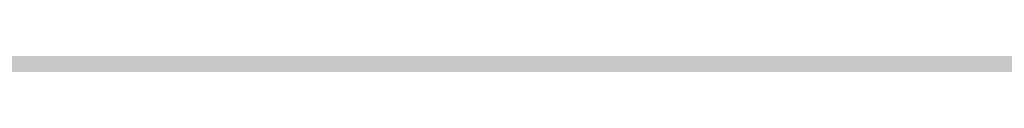
# Model space of a CAD drawing. Units: millimetres. Extents: x 0 to 2267, y 0 to 1823.
# Tile 124 of 256: x 1600.369 to 1605.705, y 1232.256 to 1232.264. Entities that reach past the tile are written whole.
import ezdxf

# ---------------------------------------------------------------- set-up
doc = ezdxf.new("R2010")
doc.units = ezdxf.units.MM
doc.header["$MEASUREMENT"] = 0
doc.layers.add('M-HATC', color=252, linetype='Continuous', lineweight=18)

msp = doc.modelspace()

# ---------------------------------------------------------------- hatches: boundary and pattern name
at = {"layer": 'M-HATC'}
h = msp.add_hatch(color=256, dxfattribs=at)
h.dxf.hatch_style = 1
h.paths.add_polyline_path([(2065.771, 1618.062, 0.236068), (2055.771, 1638.062), (1381.0868, 1638.062, 0.236068), (1371.0868, 1618.062), (1371.0868, 1603.062), (2055.771, 1603.062), (2065.771, 1603.062)])
h.paths.add_polyline_path([(2062.7718, 1550.2964), (2062.7718, 1560.2964), (1374.086, 1560.2964), (1374.086, 1550.2964), (1374.086, 1540.2964), (1384.086, 1540.2964), (1389.086, 1540.2964), (2062.7718, 1540.2964)])
h.paths.add_polyline_path([(1930.9289, 1282.7656), (1505.9289, 1282.7656), (1587.6276, 1235.5968, 0.131652), (1600.1276, 1232.2475), (1836.7302, 1232.2475, 0.131652), (1849.2302, 1235.5968)])
h.paths.add_polyline_path([(1930.9289, 1117.4171), (1905.9289, 1117.4171), (1505.9289, 1117.4171), (1505.9289, 1077.4171), (1930.9289, 1077.4171)])
h = msp.add_hatch(color=256, dxfattribs=at)
h.dxf.hatch_style = 1
h.paths.add_polyline_path([(2055.771, 1603.062), (1381.0868, 1603.062), (1381.0868, 1598.062), (2055.771, 1598.062)])
h.paths.add_polyline_path([(2055.771, 1598.062), (1381.0868, 1598.062), (1381.0868, 1593.062), (2055.771, 1593.062)])
h.paths.add_polyline_path([(2051.3074, 1536.7609), (1385.5504, 1536.7609), (1385.5504, 1526.7609), (1387.5504, 1526.7609), (1388.5366, 1525.0528), (1385.3319, 1521.2335), (1385.3319, 1521.2226), (2050.2542, 1522.7491), (2048.3212, 1525.0528), (2049.3074, 1526.7609), (2051.3074, 1526.7609)])
edge = h.paths.add_edge_path()
edge.add_arc((1847.5345, 1379.1492), 135, 222.603061, 222.890851, ccw=False)
edge.add_line((1748.1663, 1287.7656), (1683.0921, 1287.7656))
edge.add_arc((1583.7239, 1379.1492), 135, 317.109149, 317.396939, ccw=False)
edge.add_arc((1678.9686, 1290.6707), 5, 222.8909, 317.1091, ccw=False)
edge.add_arc((1774.2133, 1379.1492), 135, 222.603061, 222.890851, ccw=False)
edge.add_line((1674.8451, 1287.7656), (1609.7709, 1287.7656))
edge.add_arc((1510.4027, 1379.1492), 135, 317.109149, 317.396939, ccw=False)
edge.add_arc((1605.6474, 1290.6707), 5, 222.8909, 317.1091, ccw=False)
edge.add_arc((1700.8921, 1379.1492), 135, 222.603061, 222.890851, ccw=False)
edge.add_line((1601.5239, 1287.7656), (1536.4497, 1287.7656))
edge.add_arc((1437.0815, 1379.1492), 135, 317.109149, 317.396939, ccw=False)
edge.add_arc((1532.3262, 1290.6707), 5, 222.8909, 317.1091, ccw=False)
edge.add_arc((1627.5709, 1379.1492), 135, 222.603061, 222.890851, ccw=False)
edge.add_line((1528.2027, 1287.7656), (1505.9289, 1287.7656))
edge.add_spline(control_points=[(1505.9289, 1287.7656), (1504.2622, 1287.7656), (1504.2622, 1282.7656), (1505.9289, 1282.7656)], knot_values=[0, 0, 0, 0, 5, 5, 5, 5], degree=3, periodic=0)
edge.add_line((1505.9289, 1282.7656), (1930.9289, 1282.7656))
edge.add_spline(control_points=[(1930.9289, 1282.7656), (1932.5956, 1282.7656), (1932.5956, 1287.7656), (1930.9289, 1287.7656)], knot_values=[0, 0, 0, 0, 5, 5, 5, 5], degree=3, periodic=0)
edge.add_line((1930.9289, 1287.7656), (1903.0557, 1287.7656))
edge.add_arc((1803.6875, 1379.1492), 135, 317.109149, 317.396939, ccw=False)
edge.add_arc((1898.9322, 1290.6707), 5, 222.8909, 317.1091, ccw=False)
edge.add_arc((1994.1769, 1379.1492), 135, 222.603061, 222.890851, ccw=False)
edge.add_line((1894.8087, 1287.7656), (1829.7345, 1287.7656))
edge.add_arc((1730.3663, 1379.1492), 135, 317.109149, 317.396939, ccw=False)
edge.add_arc((1825.611, 1290.6707), 5, 222.8909, 317.1091, ccw=False)
edge.add_arc((1920.8557, 1379.1492), 135, 222.603061, 222.890851, ccw=False)
edge.add_line((1821.4875, 1287.7656), (1756.4133, 1287.7656))
edge.add_arc((1657.0451, 1379.1492), 135, 317.109149, 317.396939, ccw=False)
edge.add_arc((1752.2898, 1290.6707), 5, 222.8909, 317.1091, ccw=False)
edge = h.paths.add_edge_path()
edge.add_spline(control_points=[(1843.4289, 1227.2475), (1845.0956, 1227.2475), (1845.0956, 1232.2475), (1843.4289, 1232.2475)], knot_values=[0, 0, 0, 0, 5, 5, 5, 5], degree=3, periodic=0)
edge.add_line((1843.4289, 1232.2475), (1593.4289, 1232.2475))
edge.add_spline(control_points=[(1593.4289, 1232.2475), (1591.7622, 1232.2475), (1591.7622, 1227.2475), (1593.4289, 1227.2475)], knot_values=[0, 0, 0, 0, 5, 5, 5, 5], degree=3, periodic=0)
edge.add_line((1593.4289, 1227.2475), (1843.4289, 1227.2475))
h.paths.add_polyline_path([(1905.9289, 1127.4171), (1530.9289, 1127.4171, 0.414214), (1520.9289, 1117.4171), (1530.9289, 1117.4171), (1915.9289, 1117.4171, 0.414214)])
edge = h.paths.add_edge_path()
edge.add_arc((1397.0858, 1498.4078), 12.7299, 90.78215, 190.87871, ccw=False)
edge.add_line((1396.912, 1511.1365), (1428.0097, 1511.3488))
edge.add_line((1428.0097, 1511.3488), (1433.0097, 1511.3488))
edge.add_line((1433.0097, 1511.3488), (1434.439, 1511.3488))
edge.add_arc((1419.474, 1498.0804), 20, 41.561, 74.08211)
edge.add_line((1424.9592, 1517.3135), (1399.9351, 1517.2561))
edge.add_spline(control_points=[(1399.9307, 1517.2561), (1399.884, 1517.2131), (1399.8328, 1517.1689), (1399.7774, 1517.1236)], knot_values=[11.567499, 11.567499, 11.567499, 11.567499, 11.814249, 11.814249, 11.814249, 11.814249], degree=3, periodic=0)
edge.add_spline(control_points=[(1399.6328, 1517.0099), (1399.5831, 1516.9721), (1399.5307, 1516.9338), (1399.4759, 1516.8947)], knot_values=[11.167718, 11.167718, 11.167718, 11.167718, 11.365188, 11.365188, 11.365188, 11.365188], degree=3, periodic=0)
edge.add_spline(control_points=[(1399.3398, 1516.8001), (1399.1514, 1516.6719), (1398.9384, 1516.5377), (1398.704, 1516.3994)], knot_values=[10.376405, 10.376405, 10.376405, 10.376405, 11.00994, 11.00994, 11.00994, 11.00994], degree=3, periodic=0)
edge.add_spline(control_points=[(1398.6572, 1516.3719), (1398.5789, 1516.326), (1398.4983, 1516.2797), (1398.4155, 1516.2331)], knot_values=[10.125175, 10.125175, 10.125175, 10.125175, 10.334406, 10.334406, 10.334406, 10.334406], degree=3, periodic=0)
edge.add_spline(control_points=[(1398.2642, 1516.1487), (1398.196, 1516.1111), (1398.1263, 1516.0732), (1398.0555, 1516.0351)], knot_values=[9.832246, 9.832246, 9.832246, 9.832246, 9.999658, 9.999658, 9.999658, 9.999658], degree=3, periodic=0)
edge.add_spline(control_points=[(1397.9987, 1516.0048), (1397.7312, 1515.8621), (1397.446, 1515.7171), (1397.1466, 1515.5714)], knot_values=[9.161808, 9.161808, 9.161808, 9.161808, 9.787769, 9.787769, 9.787769, 9.787769], degree=3, periodic=0)
edge.add_spline(control_points=[(1397.1466, 1515.5714), (1396.8418, 1515.423), (1396.5222, 1515.274), (1396.1914, 1515.1262)], knot_values=[8.524455, 8.524455, 8.524455, 8.524455, 9.161808, 9.161808, 9.161808, 9.161808], degree=3, periodic=0)
edge.add_spline(control_points=[(1396.0777, 1515.0756), (1395.9854, 1515.0348), (1395.8922, 1514.994), (1395.7983, 1514.9534)], knot_values=[8.275193, 8.275193, 8.275193, 8.275193, 8.451726, 8.451726, 8.451726, 8.451726], degree=3, periodic=0)
edge.add_spline(control_points=[(1395.6018, 1514.8691), (1395.4997, 1514.8257), (1395.3968, 1514.7824), (1395.2932, 1514.7394)], knot_values=[7.962917, 7.962917, 7.962917, 7.962917, 8.152764, 8.152764, 8.152764, 8.152764], degree=3, periodic=0)
edge.add_spline(control_points=[(1395.2116, 1514.7057), (1394.8278, 1514.5475), (1394.4345, 1514.3929), (1394.0364, 1514.2442)], knot_values=[7.21254, 7.21254, 7.21254, 7.21254, 7.913148, 7.913148, 7.913148, 7.913148], degree=3, periodic=0)
edge.add_spline(control_points=[(1394.0364, 1514.2442), (1393.7076, 1514.1214), (1393.3754, 1514.0027), (1393.0427, 1513.8895)], knot_values=[6.633733, 6.633733, 6.633733, 6.633733, 7.21254, 7.21254, 7.21254, 7.21254], degree=3, periodic=0)
edge.add_spline(control_points=[(1392.8214, 1513.815), (1392.7198, 1513.7812), (1392.6181, 1513.7479), (1392.5166, 1513.7152)], knot_values=[6.328796, 6.328796, 6.328796, 6.328796, 6.505493, 6.505493, 6.505493, 6.505493], degree=3, periodic=0)
edge.add_spline(control_points=[(1392.5166, 1513.7152), (1392.3187, 1513.6515), (1392.1212, 1513.59), (1391.9244, 1513.531)], knot_values=[5.984605, 5.984605, 5.984605, 5.984605, 6.328796, 6.328796, 6.328796, 6.328796], degree=3, periodic=0)
edge.add_spline(control_points=[(1391.7915, 1513.4915), (1391.3122, 1513.3501), (1390.8384, 1513.2239), (1390.3784, 1513.1171)], knot_values=[5.066697, 5.066697, 5.066697, 5.066697, 5.907055, 5.907055, 5.907055, 5.907055], degree=3, periodic=0)
edge.add_spline(control_points=[(1390.3784, 1513.1171), (1390.1797, 1513.071), (1389.9836, 1513.0284), (1389.7907, 1512.9899)], knot_values=[4.70367, 4.70367, 4.70367, 4.70367, 5.066695, 5.066695, 5.066695, 5.066695], degree=3, periodic=0)
edge.add_spline(control_points=[(1389.422, 1512.9204), (1389.2459, 1512.8892), (1389.0729, 1512.8617), (1388.9036, 1512.8381)], knot_values=[4.130571, 4.130571, 4.130571, 4.130571, 4.469816, 4.469816, 4.469816, 4.469816], degree=3, periodic=0)
edge.add_spline(control_points=[(1388.9036, 1512.8381), (1388.591, 1512.7946), (1388.2911, 1512.7644), (1388.0071, 1512.7494)], knot_values=[3.504031, 3.504031, 3.504031, 3.504031, 4.130571, 4.130571, 4.130571, 4.130571], degree=3, periodic=0)
edge.add_spline(control_points=[(1387.9356, 1512.7459), (1387.8538, 1512.7423), (1387.7733, 1512.74), (1387.6944, 1512.739)], knot_values=[3.268866, 3.268866, 3.268866, 3.268866, 3.451164, 3.451164, 3.451164, 3.451164], degree=3, periodic=0)
edge.add_spline(control_points=[(1387.3351, 1512.7443), (1387.2076, 1512.7499), (1387.0847, 1512.7597), (1386.967, 1512.7739)], knot_values=[2.670686, 2.670686, 2.670686, 2.670686, 2.984, 2.984, 2.984, 2.984], degree=3, periodic=0)
edge.add_spline(control_points=[(1386.8327, 1512.7922), (1386.8209, 1512.7941), (1386.8092, 1512.7959), (1386.7975, 1512.7979)], knot_values=[2.516981, 2.516981, 2.516981, 2.516981, 2.549528, 2.549528, 2.549528, 2.549528], degree=3, periodic=0)
edge.add_spline(control_points=[(1386.4526, 1512.8735), (1386.4257, 1512.881), (1386.3993, 1512.889), (1386.3733, 1512.8972)], knot_values=[2.095869, 2.095869, 2.095869, 2.095869, 2.17941, 2.17941, 2.17941, 2.17941], degree=3, periodic=0)
edge.add_spline(control_points=[(1386.0691, 1513.0189), (1386.0634, 1513.0217), (1386.0577, 1513.0246), (1386.052, 1513.0275)], knot_values=[1.72453, 1.72453, 1.72453, 1.72453, 1.745933, 1.745933, 1.745933, 1.745933], degree=3, periodic=0)
edge.add_arc((1399.474, 1498.0804), 20, 131.82432, 180)
edge.add_arc((1630.3336, 1505.5484), 250.9708, 181.705176, 236.427975)
edge.add_arc((1605.3399, 1483.3044), 218.7822, 238.660829, 243.34961)
edge.add_arc((1647.0911, 1510.3592), 262.8986, 183.129836, 237.853442, ccw=False)
h.paths.add_polyline_path([(1406.5369, 1391.9644, 0.149382), (1491.5506, 1296.4418, -0.129517)], flags=17)
edge = h.paths.add_edge_path()
edge.add_arc((2037.3838, 1498.0804), 20, 0, 48.26587)
edge.add_spline(control_points=[(2050.6973, 1513.0052), (2050.6512, 1512.9847), (2050.6034, 1512.9655), (2050.5539, 1512.9477)], knot_values=[1.835652, 1.835652, 1.835652, 1.835652, 2.000781, 2.000781, 2.000781, 2.000781], degree=3, periodic=0)
edge.add_spline(control_points=[(2050.4616, 1512.9166), (2050.479, 1512.9221), (2050.4963, 1512.9277), (2050.5133, 1512.9335)], knot_values=[2.045477, 2.045477, 2.045477, 2.045477, 2.101389, 2.101389, 2.101389, 2.101389], degree=3, periodic=0)
edge.add_spline(control_points=[(2050.129, 1512.8342), (2050.1984, 1512.8473), (2050.2657, 1512.8623), (2050.3308, 1512.8792)], knot_values=[2.237629, 2.237629, 2.237629, 2.237629, 2.435841, 2.435841, 2.435841, 2.435841], degree=3, periodic=0)
edge.add_spline(control_points=[(2050.0946, 1512.8278), (2050.1061, 1512.8299), (2050.1176, 1512.832), (2050.129, 1512.8342)], knot_values=[2.435841, 2.435841, 2.435841, 2.435841, 2.468321, 2.468321, 2.468321, 2.468321], degree=3, periodic=0)
edge.add_spline(control_points=[(2049.7843, 1512.7851), (2049.8552, 1512.7922), (2049.9243, 1512.8008), (2049.9917, 1512.8109)], knot_values=[2.563852, 2.563852, 2.563852, 2.563852, 2.748541, 2.748541, 2.748541, 2.748541], degree=3, periodic=0)
edge.add_spline(control_points=[(2049.4052, 1512.7617), (2049.5364, 1512.7653), (2049.6629, 1512.773), (2049.7843, 1512.7851)], knot_values=[2.748541, 2.748541, 2.748541, 2.748541, 3.064882, 3.064882, 3.064882, 3.064882], degree=3, periodic=0)
edge.add_spline(control_points=[(2049.1698, 1512.7597), (2049.2336, 1512.7591), (2049.2965, 1512.7594), (2049.3584, 1512.7606)], knot_values=[3.102309, 3.102309, 3.102309, 3.102309, 3.2503, 3.2503, 3.2503, 3.2503], degree=3, periodic=0)
edge.add_spline(control_points=[(2048.8573, 1512.7691), (2048.9638, 1512.7638), (2049.068, 1512.7606), (2049.1698, 1512.7597)], knot_values=[3.2503, 3.2503, 3.2503, 3.2503, 3.486069, 3.486069, 3.486069, 3.486069], degree=3, periodic=0)
edge.add_spline(control_points=[(2048.6924, 1512.7789), (2048.3729, 1512.8009), (2048.0345, 1512.8411), (2047.6817, 1512.897)], knot_values=[3.606429, 3.606429, 3.606429, 3.606429, 4.2989, 4.2989, 4.2989, 4.2989], degree=3, periodic=0)
edge.add_spline(control_points=[(2047.6817, 1512.897), (2047.5458, 1512.9185), (2047.4077, 1512.9424), (2047.2678, 1512.9685)], knot_values=[4.2989, 4.2989, 4.2989, 4.2989, 4.565769, 4.565769, 4.565769, 4.565769], degree=3, periodic=0)
edge.add_spline(control_points=[(2047.2678, 1512.9685), (2047.1449, 1512.9914), (2047.0207, 1513.016), (2046.8951, 1513.0422)], knot_values=[4.565769, 4.565769, 4.565769, 4.565769, 4.799971, 4.799971, 4.799971, 4.799971], degree=3, periodic=0)
edge.add_spline(control_points=[(2046.8951, 1513.0422), (2046.5286, 1513.1188), (2046.1513, 1513.209), (2045.7676, 1513.3107)], knot_values=[4.799971, 4.799971, 4.799971, 4.799971, 5.483718, 5.483718, 5.483718, 5.483718], degree=3, periodic=0)
edge.add_spline(control_points=[(2045.7676, 1513.3107), (2045.3724, 1513.4154), (2044.9704, 1513.5322), (2044.5662, 1513.6588)], knot_values=[5.483718, 5.483718, 5.483718, 5.483718, 6.187866, 6.187866, 6.187866, 6.187866], degree=3, periodic=0)
edge.add_spline(control_points=[(2044.5662, 1513.6588), (2044.4149, 1513.7061), (2044.2633, 1513.7549), (2044.1116, 1513.8048)], knot_values=[6.187866, 6.187866, 6.187866, 6.187866, 6.451551, 6.451551, 6.451551, 6.451551], degree=3, periodic=0)
edge.add_spline(control_points=[(2044.1116, 1513.8048), (2043.9967, 1513.8427), (2043.8817, 1513.8813), (2043.7668, 1513.9205)], knot_values=[6.451551, 6.451551, 6.451551, 6.451551, 6.651434, 6.651434, 6.651434, 6.651434], degree=3, periodic=0)
edge.add_spline(control_points=[(2043.7668, 1513.9205), (2043.3716, 1514.0554), (2042.9774, 1514.1979), (2042.5886, 1514.3458)], knot_values=[6.651434, 6.651434, 6.651434, 6.651434, 7.338879, 7.338879, 7.338879, 7.338879], degree=3, periodic=0)
edge.add_spline(control_points=[(2042.5886, 1514.3458), (2042.1643, 1514.5071), (2041.7465, 1514.6749), (2041.3409, 1514.846)], knot_values=[7.338879, 7.338879, 7.338879, 7.338879, 8.089209, 8.089209, 8.089209, 8.089209], degree=3, periodic=0)
edge.add_spline(control_points=[(2041.3409, 1514.846), (2041.1028, 1514.9465), (2040.869, 1515.0481), (2040.6405, 1515.1502)], knot_values=[8.089209, 8.089209, 8.089209, 8.089209, 8.529587, 8.529587, 8.529587, 8.529587], degree=3, periodic=0)
edge.add_spline(control_points=[(2040.51, 1515.2089), (2040.0824, 1515.4022), (2039.6747, 1515.5971), (2039.295, 1515.7894)], knot_values=[8.613818, 8.613818, 8.613818, 8.613818, 9.44571, 9.44571, 9.44571, 9.44571], degree=3, periodic=0)
edge.add_spline(control_points=[(2039.295, 1515.7894), (2039.0618, 1515.9075), (2038.8391, 1516.0246), (2038.6288, 1516.1398)], knot_values=[9.44571, 9.44571, 9.44571, 9.44571, 9.956404, 9.956404, 9.956404, 9.956404], degree=3, periodic=0)
edge.add_spline(control_points=[(2038.6288, 1516.1398), (2038.5187, 1516.2001), (2038.4121, 1516.2598), (2038.309, 1516.3189)], knot_values=[9.956404, 9.956404, 9.956404, 9.956404, 10.223542, 10.223542, 10.223542, 10.223542], degree=3, periodic=0)
edge.add_spline(control_points=[(2038.309, 1516.3189), (2038.2138, 1516.3735), (2038.1216, 1516.4276), (2038.0328, 1516.481)], knot_values=[10.223542, 10.223542, 10.223542, 10.223542, 10.47051, 10.47051, 10.47051, 10.47051], degree=3, periodic=0)
edge.add_spline(control_points=[(2038.0328, 1516.481), (2037.7855, 1516.6296), (2037.5639, 1516.773), (2037.3722, 1516.909)], knot_values=[10.47051, 10.47051, 10.47051, 10.47051, 11.15767, 11.15767, 11.15767, 11.15767], degree=3, periodic=0)
edge.add_spline(control_points=[(2037.3722, 1516.909), (2037.2789, 1516.9752), (2037.1927, 1517.0396), (2037.1142, 1517.102)], knot_values=[11.15767, 11.15767, 11.15767, 11.15767, 11.49227, 11.49227, 11.49227, 11.49227], degree=3, periodic=0)
edge.add_spline(control_points=[(2036.8564, 1517.3259), (2036.9148, 1517.2692), (2036.9814, 1517.2103), (2037.0557, 1517.1492)], knot_values=[11.577341, 11.577341, 11.577341, 11.577341, 11.91035, 11.91035, 11.91035, 11.91035], degree=3, periodic=0)
edge.add_spline(control_points=[(2036.8074, 1517.3748), (2036.823, 1517.3587), (2036.8393, 1517.3424), (2036.8564, 1517.3259)], knot_values=[11.91035, 11.91035, 11.91035, 11.91035, 12.007402, 12.007402, 12.007402, 12.007402], degree=3, periodic=0)
edge.add_spline(control_points=[(2036.7017, 1517.494), (2036.7104, 1517.483), (2036.7196, 1517.4719), (2036.7291, 1517.4606)], knot_values=[12.184155, 12.184155, 12.184155, 12.184155, 12.255409, 12.255409, 12.255409, 12.255409], degree=3, periodic=0)
edge.add_spline(control_points=[(2036.6159, 1517.6205), (2036.62, 1517.613), (2036.6243, 1517.6055), (2036.6289, 1517.5979)], knot_values=[12.487913, 12.487913, 12.487913, 12.487913, 12.541035, 12.541035, 12.541035, 12.541035], degree=3, periodic=0)
edge.add_spline(control_points=[(2036.5635, 1517.786), (2036.5637, 1517.7794), (2036.5642, 1517.7726), (2036.565, 1517.7658)], knot_values=[12.911761, 12.911761, 12.911761, 12.911761, 12.968286, 12.968286, 12.968286, 12.968286], degree=3, periodic=0)
edge.add_spline(control_points=[(2036.6166, 1517.9304), (2036.6125, 1517.9259), (2036.6086, 1517.9212), (2036.6049, 1517.9165)], knot_values=[13.382527, 13.382527, 13.382527, 13.382527, 13.433791, 13.433791, 13.433791, 13.433791], degree=3, periodic=0)
edge.add_spline(control_points=[(2036.749, 1518.017), (2036.7361, 1518.0116), (2036.7239, 1518.006), (2036.7124, 1518.0002)], knot_values=[13.726299, 13.726299, 13.726299, 13.726299, 13.809928, 13.809928, 13.809928, 13.809928], degree=3, periodic=0)
edge.add_spline(control_points=[(2036.8604, 1518.0528), (2036.8386, 1518.0474), (2036.8181, 1518.0416), (2036.7988, 1518.0353)], knot_values=[13.910887, 13.910887, 13.910887, 13.910887, 14.02153, 14.02153, 14.02153, 14.02153], degree=3, periodic=0)
edge.add_line((2036.9639, 1518.0804), (2032.3838, 1518.0804))
edge.add_line((2032.3838, 1518.0804), (2027.3838, 1518.0804))
edge.add_line((2027.3838, 1518.0804), (2022.3838, 1518.0804))
edge.add_line((2022.3838, 1518.0804), (2017.3838, 1518.0804))
edge.add_arc((2017.3838, 1498.0804), 20, 90, 138.439)
edge.add_line((2002.4188, 1511.3488), (2003.8481, 1511.3488))
edge.add_line((2003.8481, 1511.3488), (2008.8481, 1511.3488))
edge.add_line((2008.8481, 1511.3488), (2039.772, 1511.1377))
edge.add_arc((2039.772, 1498.4078), 12.7299, -10.87871, 90, ccw=False)
edge.add_arc((1789.7668, 1510.3592), 262.8986, 302.146558, 356.870164, ccw=False)
edge.add_arc((1831.5179, 1483.3044), 218.7822, 296.65039, 301.339171)
edge.add_arc((1806.5242, 1505.5484), 250.9708, 303.572025, 358.294824)
h.paths.add_polyline_path([(2030.321, 1391.9644, -0.129517), (1945.3072, 1296.4418, 0.149382)], flags=17)
edge = h.paths.add_edge_path()
edge.add_spline(control_points=[(2037.2464, 1518.0821), (2037.2898, 1518.081), (2037.3355, 1518.0804), (2037.3838, 1518.0804)], knot_values=[0.000012, 0.000012, 0.000012, 0.000012, 0.144754, 0.144754, 0.144754, 0.144754], degree=3, periodic=0)
edge.add_line((2037.3357, 1518.0804), (2037.0096, 1518.0804))
edge.add_spline(control_points=[(2037.0096, 1518.0804), (2036.9822, 1518.0768), (2036.956, 1518.0727), (2036.9312, 1518.0681)], knot_values=[14.13465, 14.13465, 14.13465, 14.13465, 14.247197, 14.247197, 14.247197, 14.247197], degree=3, periodic=0)
edge.add_spline(control_points=[(2036.9312, 1518.0681), (2036.9276, 1518.0674), (2036.9241, 1518.0667), (2036.9205, 1518.0661)], knot_values=[14.118315, 14.118315, 14.118315, 14.118315, 14.13465, 14.13465, 14.13465, 14.13465], degree=3, periodic=0)
edge.add_spline(control_points=[(2036.9205, 1518.0661), (2036.9118, 1518.0644), (2036.9032, 1518.0626), (2036.8948, 1518.0608)], knot_values=[14.078086, 14.078086, 14.078086, 14.078086, 14.118315, 14.118315, 14.118315, 14.118315], degree=3, periodic=0)
edge.add_spline(control_points=[(2036.8948, 1518.0608), (2036.883, 1518.0583), (2036.8716, 1518.0556), (2036.8604, 1518.0528)], knot_values=[14.02153, 14.02153, 14.02153, 14.02153, 14.078086, 14.078086, 14.078086, 14.078086], degree=3, periodic=0)
edge.add_spline(control_points=[(2036.8604, 1518.0528), (2036.8386, 1518.0474), (2036.8181, 1518.0416), (2036.7988, 1518.0353)], knot_values=[13.910887, 13.910887, 13.910887, 13.910887, 14.02153, 14.02153, 14.02153, 14.02153], degree=3, periodic=0)
edge.add_spline(control_points=[(2036.7988, 1518.0353), (2036.7981, 1518.035), (2036.7974, 1518.0348), (2036.7967, 1518.0346)], knot_values=[13.906906, 13.906906, 13.906906, 13.906906, 13.910887, 13.910887, 13.910887, 13.910887], degree=3, periodic=0)
edge.add_spline(control_points=[(2036.7967, 1518.0346), (2036.7882, 1518.0318), (2036.7799, 1518.0289), (2036.7719, 1518.0259)], knot_values=[13.857826, 13.857826, 13.857826, 13.857826, 13.906906, 13.906906, 13.906906, 13.906906], degree=3, periodic=0)
edge.add_spline(control_points=[(2036.7719, 1518.0259), (2036.764, 1518.023), (2036.7564, 1518.02), (2036.749, 1518.017)], knot_values=[13.809928, 13.809928, 13.809928, 13.809928, 13.857826, 13.857826, 13.857826, 13.857826], degree=3, periodic=0)
edge.add_spline(control_points=[(2036.749, 1518.017), (2036.7361, 1518.0116), (2036.7239, 1518.006), (2036.7124, 1518.0002)], knot_values=[13.726299, 13.726299, 13.726299, 13.726299, 13.809928, 13.809928, 13.809928, 13.809928], degree=3, periodic=0)
edge.add_spline(control_points=[(2036.7124, 1518.0002), (2036.7121, 1518), (2036.7118, 1517.9999), (2036.7115, 1517.9997)], knot_values=[13.723993, 13.723993, 13.723993, 13.723993, 13.726299, 13.726299, 13.726299, 13.726299], degree=3, periodic=0)
edge.add_spline(control_points=[(2036.7115, 1517.9997), (2036.7063, 1517.9971), (2036.7013, 1517.9944), (2036.6965, 1517.9917)], knot_values=[13.686536, 13.686536, 13.686536, 13.686536, 13.723993, 13.723993, 13.723993, 13.723993], degree=3, periodic=0)
edge.add_spline(control_points=[(2036.6965, 1517.9917), (2036.6919, 1517.9891), (2036.6874, 1517.9865), (2036.6831, 1517.9839)], knot_values=[13.651251, 13.651251, 13.651251, 13.651251, 13.686536, 13.686536, 13.686536, 13.686536], degree=3, periodic=0)
edge.add_spline(control_points=[(2036.6831, 1517.9839), (2036.6764, 1517.9798), (2036.67, 1517.9757), (2036.6639, 1517.9714)], knot_values=[13.596804, 13.596804, 13.596804, 13.596804, 13.651251, 13.651251, 13.651251, 13.651251], degree=3, periodic=0)
edge.add_spline(control_points=[(2036.6639, 1517.9714), (2036.6636, 1517.9712), (2036.6633, 1517.9709), (2036.6629, 1517.9707)], knot_values=[13.593956, 13.593956, 13.593956, 13.593956, 13.596804, 13.596804, 13.596804, 13.596804], degree=3, periodic=0)
edge.add_spline(control_points=[(2036.6629, 1517.9707), (2036.6603, 1517.9689), (2036.6577, 1517.967), (2036.6552, 1517.9651)], knot_values=[13.570322, 13.570322, 13.570322, 13.570322, 13.593956, 13.593956, 13.593956, 13.593956], degree=3, periodic=0)
edge.add_spline(control_points=[(2036.6552, 1517.9651), (2036.6525, 1517.9631), (2036.6499, 1517.9611), (2036.6474, 1517.9591)], knot_values=[13.545477, 13.545477, 13.545477, 13.545477, 13.570322, 13.570322, 13.570322, 13.570322], degree=3, periodic=0)
edge.add_spline(control_points=[(2036.6474, 1517.9591), (2036.6472, 1517.9589), (2036.6471, 1517.9588), (2036.6469, 1517.9587)], knot_values=[13.543931, 13.543931, 13.543931, 13.543931, 13.545477, 13.545477, 13.545477, 13.545477], degree=3, periodic=0)
edge.add_spline(control_points=[(2036.6469, 1517.9587), (2036.6412, 1517.9541), (2036.6358, 1517.9494), (2036.6307, 1517.9447)], knot_values=[13.488237, 13.488237, 13.488237, 13.488237, 13.543931, 13.543931, 13.543931, 13.543931], degree=3, periodic=0)
edge.add_spline(control_points=[(2036.6307, 1517.9447), (2036.6282, 1517.9423), (2036.6257, 1517.9399), (2036.6233, 1517.9374)], knot_values=[13.460307, 13.460307, 13.460307, 13.460307, 13.488237, 13.488237, 13.488237, 13.488237], degree=3, periodic=0)
edge.add_spline(control_points=[(2036.6233, 1517.9374), (2036.6215, 1517.9356), (2036.6198, 1517.9338), (2036.6181, 1517.932)], knot_values=[13.439712, 13.439712, 13.439712, 13.439712, 13.460307, 13.460307, 13.460307, 13.460307], degree=3, periodic=0)
edge.add_spline(control_points=[(2036.6181, 1517.932), (2036.6176, 1517.9315), (2036.6171, 1517.9309), (2036.6166, 1517.9304)], knot_values=[13.433791, 13.433791, 13.433791, 13.433791, 13.439712, 13.439712, 13.439712, 13.439712], degree=3, periodic=0)
edge.add_spline(control_points=[(2036.6166, 1517.9304), (2036.6125, 1517.9259), (2036.6086, 1517.9212), (2036.6049, 1517.9165)], knot_values=[13.382527, 13.382527, 13.382527, 13.382527, 13.433791, 13.433791, 13.433791, 13.433791], degree=3, periodic=0)
edge.add_spline(control_points=[(2036.6049, 1517.9165), (2036.6026, 1517.9135), (2036.6004, 1517.9104), (2036.5982, 1517.9074)], knot_values=[13.350017, 13.350017, 13.350017, 13.350017, 13.382527, 13.382527, 13.382527, 13.382527], degree=3, periodic=0)
edge.add_spline(control_points=[(2036.5982, 1517.9074), (2036.5972, 1517.9059), (2036.5962, 1517.9043), (2036.5952, 1517.9028)], knot_values=[13.333922, 13.333922, 13.333922, 13.333922, 13.350017, 13.350017, 13.350017, 13.350017], degree=3, periodic=0)
edge.add_spline(control_points=[(2036.5952, 1517.9028), (2036.5945, 1517.9018), (2036.5939, 1517.9009), (2036.5933, 1517.8999)], knot_values=[13.323828, 13.323828, 13.323828, 13.323828, 13.333922, 13.333922, 13.333922, 13.333922], degree=3, periodic=0)
edge.add_spline(control_points=[(2036.5933, 1517.8999), (2036.5905, 1517.8955), (2036.5879, 1517.8909), (2036.5855, 1517.8864)], knot_values=[13.277545, 13.277545, 13.277545, 13.277545, 13.323828, 13.323828, 13.323828, 13.323828], degree=3, periodic=0)
edge.add_spline(control_points=[(2036.5855, 1517.8864), (2036.5836, 1517.8827), (2036.5817, 1517.8789), (2036.5801, 1517.8751)], knot_values=[13.240119, 13.240119, 13.240119, 13.240119, 13.277545, 13.277545, 13.277545, 13.277545], degree=3, periodic=0)
edge.add_spline(control_points=[(2036.5801, 1517.8751), (2036.5795, 1517.8739), (2036.579, 1517.8727), (2036.5785, 1517.8715)], knot_values=[13.228211, 13.228211, 13.228211, 13.228211, 13.240119, 13.240119, 13.240119, 13.240119], degree=3, periodic=0)
edge.add_spline(control_points=[(2036.5785, 1517.8715), (2036.578, 1517.8702), (2036.5774, 1517.869), (2036.5769, 1517.8677)], knot_values=[13.215717, 13.215717, 13.215717, 13.215717, 13.228211, 13.228211, 13.228211, 13.228211], degree=3, periodic=0)
edge.add_spline(control_points=[(2036.5769, 1517.8677), (2036.5755, 1517.864), (2036.5741, 1517.8603), (2036.5729, 1517.8565)], knot_values=[13.179847, 13.179847, 13.179847, 13.179847, 13.215717, 13.215717, 13.215717, 13.215717], degree=3, periodic=0)
edge.add_spline(control_points=[(2036.5729, 1517.8565), (2036.5713, 1517.8515), (2036.5699, 1517.8464), (2036.5687, 1517.8413)], knot_values=[13.132017, 13.132017, 13.132017, 13.132017, 13.179847, 13.179847, 13.179847, 13.179847], degree=3, periodic=0)
edge.add_spline(control_points=[(2036.5687, 1517.8413), (2036.5684, 1517.8402), (2036.5682, 1517.8392), (2036.568, 1517.8382)], knot_values=[13.122482, 13.122482, 13.122482, 13.122482, 13.132017, 13.132017, 13.132017, 13.132017], degree=3, periodic=0)
edge.add_spline(control_points=[(2036.568, 1517.8382), (2036.5676, 1517.8363), (2036.5672, 1517.8345), (2036.5669, 1517.8327)], knot_values=[13.105592, 13.105592, 13.105592, 13.105592, 13.122482, 13.122482, 13.122482, 13.122482], degree=3, periodic=0)
edge.add_spline(control_points=[(2036.5669, 1517.8327), (2036.5662, 1517.8292), (2036.5657, 1517.8257), (2036.5652, 1517.8222)], knot_values=[13.074063, 13.074063, 13.074063, 13.074063, 13.105592, 13.105592, 13.105592, 13.105592], degree=3, periodic=0)
edge.add_spline(control_points=[(2036.5652, 1517.8222), (2036.5652, 1517.8222), (2036.5652, 1517.8222), (2036.5652, 1517.8222)], knot_values=[13.074043, 13.074043, 13.074043, 13.074043, 13.074063, 13.074063, 13.074063, 13.074063], degree=3, periodic=0)
edge.add_spline(control_points=[(2036.5652, 1517.8222), (2036.5644, 1517.8164), (2036.5639, 1517.8106), (2036.5636, 1517.8046)], knot_values=[13.021884, 13.021884, 13.021884, 13.021884, 13.074043, 13.074043, 13.074043, 13.074043], degree=3, periodic=0)
edge.add_spline(control_points=[(2036.5636, 1517.8046), (2036.5636, 1517.804), (2036.5636, 1517.8034), (2036.5635, 1517.8028)], knot_values=[13.01674, 13.01674, 13.01674, 13.01674, 13.021884, 13.021884, 13.021884, 13.021884], degree=3, periodic=0)
edge.add_spline(control_points=[(2036.5635, 1517.8028), (2036.5634, 1517.8005), (2036.5634, 1517.7982), (2036.5634, 1517.7958)], knot_values=[12.996438, 12.996438, 12.996438, 12.996438, 13.01674, 13.01674, 13.01674, 13.01674], degree=3, periodic=0)
edge.add_spline(control_points=[(2036.5634, 1517.7958), (2036.5633, 1517.7926), (2036.5634, 1517.7893), (2036.5635, 1517.786)], knot_values=[12.968286, 12.968286, 12.968286, 12.968286, 12.996438, 12.996438, 12.996438, 12.996438], degree=3, periodic=0)
edge.add_spline(control_points=[(2036.5635, 1517.786), (2036.5637, 1517.7794), (2036.5642, 1517.7726), (2036.565, 1517.7658)], knot_values=[12.911761, 12.911761, 12.911761, 12.911761, 12.968286, 12.968286, 12.968286, 12.968286], degree=3, periodic=0)
edge.add_spline(control_points=[(2036.565, 1517.7658), (2036.565, 1517.7657), (2036.565, 1517.7656), (2036.565, 1517.7656)], knot_values=[12.911017, 12.911017, 12.911017, 12.911017, 12.911761, 12.911761, 12.911761, 12.911761], degree=3, periodic=0)
edge.add_spline(control_points=[(2036.565, 1517.7656), (2036.5654, 1517.7625), (2036.5658, 1517.7593), (2036.5663, 1517.7562)], knot_values=[12.88528, 12.88528, 12.88528, 12.88528, 12.911017, 12.911017, 12.911017, 12.911017], degree=3, periodic=0)
edge.add_spline(control_points=[(2036.5663, 1517.7562), (2036.5667, 1517.7534), (2036.5672, 1517.7506), (2036.5677, 1517.7478)], knot_values=[12.862519, 12.862519, 12.862519, 12.862519, 12.88528, 12.88528, 12.88528, 12.88528], degree=3, periodic=0)
edge.add_spline(control_points=[(2036.5677, 1517.7478), (2036.5678, 1517.7474), (2036.5679, 1517.7469), (2036.568, 1517.7465)], knot_values=[12.858885, 12.858885, 12.858885, 12.858885, 12.862519, 12.862519, 12.862519, 12.862519], degree=3, periodic=0)
edge.add_spline(control_points=[(2036.568, 1517.7465), (2036.5692, 1517.7399), (2036.5707, 1517.7332), (2036.5724, 1517.7264)], knot_values=[12.8053, 12.8053, 12.8053, 12.8053, 12.858885, 12.858885, 12.858885, 12.858885], degree=3, periodic=0)
edge.add_spline(control_points=[(2036.5724, 1517.7264), (2036.5734, 1517.7226), (2036.5745, 1517.7187), (2036.5756, 1517.7149)], knot_values=[12.775176, 12.775176, 12.775176, 12.775176, 12.8053, 12.8053, 12.8053, 12.8053], degree=3, periodic=0)
edge.add_spline(control_points=[(2036.5756, 1517.7149), (2036.5763, 1517.7125), (2036.577, 1517.7102), (2036.5778, 1517.7078)], knot_values=[12.756759, 12.756759, 12.756759, 12.756759, 12.775176, 12.775176, 12.775176, 12.775176], degree=3, periodic=0)
edge.add_spline(control_points=[(2036.5778, 1517.7078), (2036.5781, 1517.7067), (2036.5784, 1517.7057), (2036.5787, 1517.7047)], knot_values=[12.748742, 12.748742, 12.748742, 12.748742, 12.756759, 12.756759, 12.756759, 12.756759], degree=3, periodic=0)
edge.add_spline(control_points=[(2036.5787, 1517.7047), (2036.5808, 1517.6983), (2036.5831, 1517.6919), (2036.5856, 1517.6854)], knot_values=[12.69959, 12.69959, 12.69959, 12.69959, 12.748742, 12.748742, 12.748742, 12.748742], degree=3, periodic=0)
edge.add_spline(control_points=[(2036.5856, 1517.6854), (2036.5876, 1517.68), (2036.5898, 1517.6746), (2036.5921, 1517.6692)], knot_values=[12.659038, 12.659038, 12.659038, 12.659038, 12.69959, 12.69959, 12.69959, 12.69959], degree=3, periodic=0)
edge.add_spline(control_points=[(2036.5921, 1517.6692), (2036.594, 1517.6648), (2036.5959, 1517.6605), (2036.5979, 1517.6561)], knot_values=[12.626806, 12.626806, 12.626806, 12.626806, 12.659038, 12.659038, 12.659038, 12.659038], degree=3, periodic=0)
edge.add_spline(control_points=[(2036.5979, 1517.6561), (2036.5984, 1517.6551), (2036.5989, 1517.6541), (2036.5993, 1517.6531)], knot_values=[12.619394, 12.619394, 12.619394, 12.619394, 12.626806, 12.626806, 12.626806, 12.626806], degree=3, periodic=0)
edge.add_spline(control_points=[(2036.5993, 1517.6531), (2036.6043, 1517.6424), (2036.6099, 1517.6315), (2036.6159, 1517.6205)], knot_values=[12.541039, 12.541039, 12.541039, 12.541039, 12.619394, 12.619394, 12.619394, 12.619394], degree=3, periodic=0)
edge.add_spline(control_points=[(2036.6159, 1517.6205), (2036.6159, 1517.6205), (2036.6159, 1517.6205), (2036.6159, 1517.6205)], knot_values=[12.541035, 12.541035, 12.541035, 12.541035, 12.541039, 12.541039, 12.541039, 12.541039], degree=3, periodic=0)
edge.add_spline(control_points=[(2036.6159, 1517.6205), (2036.62, 1517.613), (2036.6243, 1517.6055), (2036.6289, 1517.5979)], knot_values=[12.487913, 12.487913, 12.487913, 12.487913, 12.541035, 12.541035, 12.541035, 12.541035], degree=3, periodic=0)
edge.add_spline(control_points=[(2036.6289, 1517.5979), (2036.6326, 1517.5916), (2036.6365, 1517.5853), (2036.6406, 1517.5789)], knot_values=[12.443982, 12.443982, 12.443982, 12.443982, 12.487913, 12.487913, 12.487913, 12.487913], degree=3, periodic=0)
edge.add_spline(control_points=[(2036.6406, 1517.5789), (2036.6414, 1517.5776), (2036.6423, 1517.5763), (2036.6431, 1517.5749)], knot_values=[12.434996, 12.434996, 12.434996, 12.434996, 12.443982, 12.443982, 12.443982, 12.443982], degree=3, periodic=0)
edge.add_spline(control_points=[(2036.6431, 1517.5749), (2036.6531, 1517.5596), (2036.6639, 1517.5439), (2036.6756, 1517.528)], knot_values=[12.329647, 12.329647, 12.329647, 12.329647, 12.434996, 12.434996, 12.434996, 12.434996], degree=3, periodic=0)
edge.add_spline(control_points=[(2036.6756, 1517.528), (2036.6839, 1517.5168), (2036.6925, 1517.5055), (2036.7017, 1517.494)], knot_values=[12.255409, 12.255409, 12.255409, 12.255409, 12.329647, 12.329647, 12.329647, 12.329647], degree=3, periodic=0)
edge.add_spline(control_points=[(2036.7017, 1517.494), (2036.7104, 1517.483), (2036.7196, 1517.4719), (2036.7291, 1517.4606)], knot_values=[12.184155, 12.184155, 12.184155, 12.184155, 12.255409, 12.255409, 12.255409, 12.255409], degree=3, periodic=0)
edge.add_spline(control_points=[(2036.7291, 1517.4606), (2036.7436, 1517.4435), (2036.759, 1517.4262), (2036.7753, 1517.4085)], knot_values=[12.075961, 12.075961, 12.075961, 12.075961, 12.184155, 12.184155, 12.184155, 12.184155], degree=3, periodic=0)
edge.add_spline(control_points=[(2036.7753, 1517.4085), (2036.7763, 1517.4075), (2036.7773, 1517.4064), (2036.7783, 1517.4054)], knot_values=[12.069502, 12.069502, 12.069502, 12.069502, 12.075961, 12.075961, 12.075961, 12.075961], degree=3, periodic=0)
edge.add_spline(control_points=[(2036.7783, 1517.4054), (2036.7877, 1517.3953), (2036.7974, 1517.385), (2036.8074, 1517.3748)], knot_values=[12.007402, 12.007402, 12.007402, 12.007402, 12.069502, 12.069502, 12.069502, 12.069502], degree=3, periodic=0)
edge.add_spline(control_points=[(2036.8074, 1517.3748), (2036.823, 1517.3587), (2036.8393, 1517.3424), (2036.8564, 1517.3259)], knot_values=[11.91035, 11.91035, 11.91035, 11.91035, 12.007402, 12.007402, 12.007402, 12.007402], degree=3, periodic=0)
edge.add_spline(control_points=[(2036.8564, 1517.3259), (2036.9148, 1517.2692), (2036.9814, 1517.2103), (2037.0557, 1517.1492)], knot_values=[11.577341, 11.577341, 11.577341, 11.577341, 11.91035, 11.91035, 11.91035, 11.91035], degree=3, periodic=0)
edge.add_spline(control_points=[(2037.0557, 1517.1492), (2037.0747, 1517.1336), (2037.0942, 1517.1179), (2037.1142, 1517.102)], knot_values=[11.49227, 11.49227, 11.49227, 11.49227, 11.577341, 11.577341, 11.577341, 11.577341], degree=3, periodic=0)
edge.add_spline(control_points=[(2037.1142, 1517.102), (2037.1927, 1517.0396), (2037.2789, 1516.9752), (2037.3722, 1516.909)], knot_values=[11.15767, 11.15767, 11.15767, 11.15767, 11.49227, 11.49227, 11.49227, 11.49227], degree=3, periodic=0)
edge.add_spline(control_points=[(2037.3722, 1516.909), (2037.5639, 1516.773), (2037.7855, 1516.6296), (2038.0328, 1516.481)], knot_values=[10.47051, 10.47051, 10.47051, 10.47051, 11.15767, 11.15767, 11.15767, 11.15767], degree=3, periodic=0)
edge.add_spline(control_points=[(2038.0328, 1516.481), (2038.1216, 1516.4276), (2038.2138, 1516.3735), (2038.309, 1516.3189)], knot_values=[10.223542, 10.223542, 10.223542, 10.223542, 10.47051, 10.47051, 10.47051, 10.47051], degree=3, periodic=0)
edge.add_spline(control_points=[(2038.309, 1516.3189), (2038.4121, 1516.2598), (2038.5187, 1516.2001), (2038.6288, 1516.1398)], knot_values=[9.956404, 9.956404, 9.956404, 9.956404, 10.223542, 10.223542, 10.223542, 10.223542], degree=3, periodic=0)
edge.add_spline(control_points=[(2038.6288, 1516.1398), (2038.8391, 1516.0246), (2039.0618, 1515.9075), (2039.295, 1515.7894)], knot_values=[9.44571, 9.44571, 9.44571, 9.44571, 9.956404, 9.956404, 9.956404, 9.956404], degree=3, periodic=0)
edge.add_spline(control_points=[(2039.295, 1515.7894), (2039.6747, 1515.5971), (2040.0824, 1515.4022), (2040.51, 1515.2089)], knot_values=[8.613818, 8.613818, 8.613818, 8.613818, 9.44571, 9.44571, 9.44571, 9.44571], degree=3, periodic=0)
edge.add_spline(control_points=[(2040.51, 1515.2089), (2040.5533, 1515.1893), (2040.5968, 1515.1697), (2040.6405, 1515.1502)], knot_values=[8.529587, 8.529587, 8.529587, 8.529587, 8.613818, 8.613818, 8.613818, 8.613818], degree=3, periodic=0)
edge.add_spline(control_points=[(2040.6405, 1515.1502), (2040.869, 1515.0481), (2041.1028, 1514.9465), (2041.3409, 1514.846)], knot_values=[8.089209, 8.089209, 8.089209, 8.089209, 8.529587, 8.529587, 8.529587, 8.529587], degree=3, periodic=0)
edge.add_spline(control_points=[(2041.3409, 1514.846), (2041.7465, 1514.6749), (2042.1643, 1514.5071), (2042.5886, 1514.3458)], knot_values=[7.338879, 7.338879, 7.338879, 7.338879, 8.089209, 8.089209, 8.089209, 8.089209], degree=3, periodic=0)
edge.add_spline(control_points=[(2042.5886, 1514.3458), (2042.9774, 1514.1979), (2043.3716, 1514.0554), (2043.7668, 1513.9205)], knot_values=[6.651434, 6.651434, 6.651434, 6.651434, 7.338879, 7.338879, 7.338879, 7.338879], degree=3, periodic=0)
edge.add_spline(control_points=[(2043.7668, 1513.9205), (2043.8817, 1513.8813), (2043.9967, 1513.8427), (2044.1116, 1513.8048)], knot_values=[6.451551, 6.451551, 6.451551, 6.451551, 6.651434, 6.651434, 6.651434, 6.651434], degree=3, periodic=0)
edge.add_spline(control_points=[(2044.1116, 1513.8048), (2044.2633, 1513.7549), (2044.4149, 1513.7061), (2044.5662, 1513.6588)], knot_values=[6.187866, 6.187866, 6.187866, 6.187866, 6.451551, 6.451551, 6.451551, 6.451551], degree=3, periodic=0)
edge.add_spline(control_points=[(2044.5662, 1513.6588), (2044.9704, 1513.5322), (2045.3724, 1513.4154), (2045.7676, 1513.3107)], knot_values=[5.483718, 5.483718, 5.483718, 5.483718, 6.187866, 6.187866, 6.187866, 6.187866], degree=3, periodic=0)
edge.add_spline(control_points=[(2045.7676, 1513.3107), (2046.1513, 1513.209), (2046.5286, 1513.1188), (2046.8951, 1513.0422)], knot_values=[4.799971, 4.799971, 4.799971, 4.799971, 5.483718, 5.483718, 5.483718, 5.483718], degree=3, periodic=0)
edge.add_spline(control_points=[(2046.8951, 1513.0422), (2047.0207, 1513.016), (2047.1449, 1512.9914), (2047.2678, 1512.9685)], knot_values=[4.565769, 4.565769, 4.565769, 4.565769, 4.799971, 4.799971, 4.799971, 4.799971], degree=3, periodic=0)
edge.add_spline(control_points=[(2047.2678, 1512.9685), (2047.4077, 1512.9424), (2047.5458, 1512.9185), (2047.6817, 1512.897)], knot_values=[4.2989, 4.2989, 4.2989, 4.2989, 4.565769, 4.565769, 4.565769, 4.565769], degree=3, periodic=0)
edge.add_spline(control_points=[(2047.6817, 1512.897), (2048.0345, 1512.8411), (2048.3729, 1512.8009), (2048.6924, 1512.7789)], knot_values=[3.606429, 3.606429, 3.606429, 3.606429, 4.2989, 4.2989, 4.2989, 4.2989], degree=3, periodic=0)
edge.add_spline(control_points=[(2048.6924, 1512.7789), (2048.7479, 1512.7751), (2048.8029, 1512.7718), (2048.8573, 1512.7691)], knot_values=[3.486069, 3.486069, 3.486069, 3.486069, 3.606429, 3.606429, 3.606429, 3.606429], degree=3, periodic=0)
edge.add_spline(control_points=[(2048.8573, 1512.7691), (2048.9638, 1512.7638), (2049.068, 1512.7606), (2049.1698, 1512.7597)], knot_values=[3.2503, 3.2503, 3.2503, 3.2503, 3.486069, 3.486069, 3.486069, 3.486069], degree=3, periodic=0)
edge.add_spline(control_points=[(2049.1698, 1512.7597), (2049.2336, 1512.7591), (2049.2965, 1512.7594), (2049.3584, 1512.7606)], knot_values=[3.102309, 3.102309, 3.102309, 3.102309, 3.2503, 3.2503, 3.2503, 3.2503], degree=3, periodic=0)
edge.add_spline(control_points=[(2049.3584, 1512.7606), (2049.3741, 1512.7609), (2049.3897, 1512.7613), (2049.4052, 1512.7617)], knot_values=[3.064882, 3.064882, 3.064882, 3.064882, 3.102309, 3.102309, 3.102309, 3.102309], degree=3, periodic=0)
edge.add_spline(control_points=[(2049.4052, 1512.7617), (2049.5364, 1512.7653), (2049.6629, 1512.773), (2049.7843, 1512.7851)], knot_values=[2.748541, 2.748541, 2.748541, 2.748541, 3.064882, 3.064882, 3.064882, 3.064882], degree=3, periodic=0)
edge.add_spline(control_points=[(2049.7843, 1512.7851), (2049.8552, 1512.7922), (2049.9243, 1512.8008), (2049.9917, 1512.8109)], knot_values=[2.563852, 2.563852, 2.563852, 2.563852, 2.748541, 2.748541, 2.748541, 2.748541], degree=3, periodic=0)
edge.add_spline(control_points=[(2049.9917, 1512.8109), (2050.0265, 1512.8161), (2050.0608, 1512.8218), (2050.0946, 1512.8278)], knot_values=[2.468321, 2.468321, 2.468321, 2.468321, 2.563852, 2.563852, 2.563852, 2.563852], degree=3, periodic=0)
edge.add_spline(control_points=[(2050.0946, 1512.8278), (2050.1061, 1512.8299), (2050.1176, 1512.832), (2050.129, 1512.8342)], knot_values=[2.435841, 2.435841, 2.435841, 2.435841, 2.468321, 2.468321, 2.468321, 2.468321], degree=3, periodic=0)
edge.add_spline(control_points=[(2050.129, 1512.8342), (2050.1984, 1512.8473), (2050.2657, 1512.8623), (2050.3308, 1512.8792)], knot_values=[2.237629, 2.237629, 2.237629, 2.237629, 2.435841, 2.435841, 2.435841, 2.435841], degree=3, periodic=0)
edge.add_spline(control_points=[(2050.3308, 1512.8792), (2050.3754, 1512.8908), (2050.4191, 1512.9032), (2050.4616, 1512.9166)], knot_values=[2.101389, 2.101389, 2.101389, 2.101389, 2.237629, 2.237629, 2.237629, 2.237629], degree=3, periodic=0)
edge.add_spline(control_points=[(2050.4616, 1512.9166), (2050.479, 1512.9221), (2050.4963, 1512.9277), (2050.5133, 1512.9335)], knot_values=[2.045477, 2.045477, 2.045477, 2.045477, 2.101389, 2.101389, 2.101389, 2.101389], degree=3, periodic=0)
edge.add_spline(control_points=[(2050.5133, 1512.9335), (2050.527, 1512.9382), (2050.5405, 1512.9429), (2050.5539, 1512.9477)], knot_values=[2.000781, 2.000781, 2.000781, 2.000781, 2.045477, 2.045477, 2.045477, 2.045477], degree=3, periodic=0)
edge.add_spline(control_points=[(2050.5539, 1512.9477), (2050.6034, 1512.9655), (2050.6512, 1512.9847), (2050.6973, 1513.0052)], knot_values=[1.835652, 1.835652, 1.835652, 1.835652, 2.000781, 2.000781, 2.000781, 2.000781], degree=3, periodic=0)
edge.add_arc((2037.3838, 1498.0804), 20, 48.26587, 90.12993)
edge = h.paths.add_edge_path(flags=16)
edge.add_spline(control_points=[(1386.1389, 1512.9859), (1388.92, 1511.7395), (1398.0387, 1515.5187), (1399.9307, 1517.2561)], knot_values=[1.831046, 1.831046, 1.831046, 1.831046, 11.814249, 11.814249, 11.814249, 11.814249], degree=3, periodic=0)
edge.add_line((1399.9307, 1517.2561), (1393.7435, 1517.2419))
edge.add_arc((1399.474, 1498.0804), 20, 106.6501, 131.8173)

doc.saveas('drawing.dxf')
